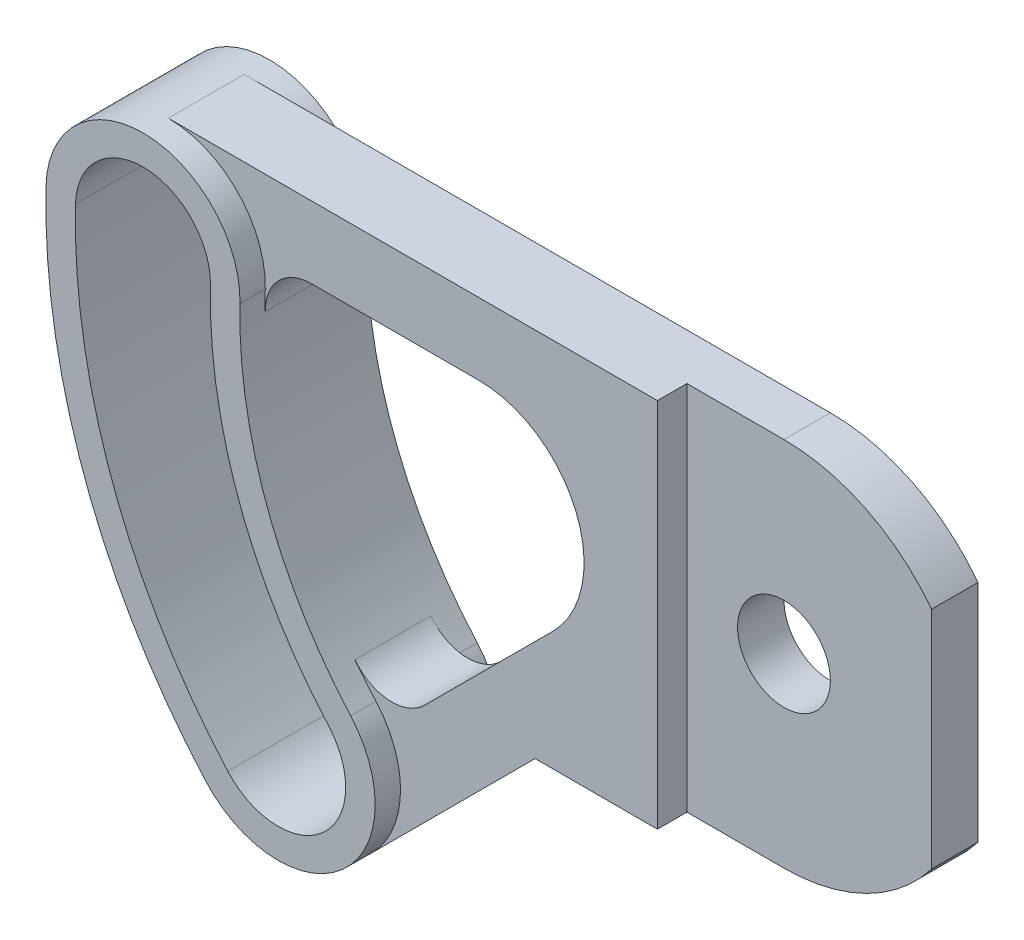
ISO-10303-21;
HEADER;
FILE_DESCRIPTION(('STEP AP214'),'2;1');
FILE_NAME('part.step','',(''),(''),'','','');
FILE_SCHEMA(('AUTOMOTIVE_DESIGN { 1 0 10303 214 1 1 1 1 }'));
ENDSEC;
DATA;
#1=APPLICATION_CONTEXT('core data for automotive mechanical design processes');
#2=APPLICATION_PROTOCOL_DEFINITION('international standard','automotive_design',2000,#1);
#3=PRODUCT_CONTEXT('',#1,'mechanical');
#4=PRODUCT('Part','Part','',(#3));
#5=PRODUCT_RELATED_PRODUCT_CATEGORY('part','',(#4));
#6=PRODUCT_DEFINITION_FORMATION('','',#4);
#7=PRODUCT_DEFINITION_CONTEXT('part definition',#1,'design');
#8=PRODUCT_DEFINITION('design','',#6,#7);
#9=PRODUCT_DEFINITION_SHAPE('','',#8);
#10=(LENGTH_UNIT() NAMED_UNIT(*) SI_UNIT(.MILLI.,.METRE.));
#11=(NAMED_UNIT(*) PLANE_ANGLE_UNIT() SI_UNIT($,.RADIAN.));
#12=(NAMED_UNIT(*) SI_UNIT($,.STERADIAN.) SOLID_ANGLE_UNIT());
#13=UNCERTAINTY_MEASURE_WITH_UNIT(LENGTH_MEASURE(1.E-05),#10,'distance_accuracy_value','');
#14=(GEOMETRIC_REPRESENTATION_CONTEXT(3) GLOBAL_UNCERTAINTY_ASSIGNED_CONTEXT((#13)) GLOBAL_UNIT_ASSIGNED_CONTEXT((#10,
#11,#12)) REPRESENTATION_CONTEXT('',''));
#15=CARTESIAN_POINT('',(0.,0.,0.));
#16=DIRECTION('',(0.,0.,1.));
#17=DIRECTION('',(1.,0.,0.));
#18=AXIS2_PLACEMENT_3D('',#15,#16,#17);
#19=CARTESIAN_POINT('',(-12.,18.,15.));
#20=DIRECTION('',(0.,0.,-1.));
#21=DIRECTION('',(-1.,0.,0.));
#22=AXIS2_PLACEMENT_3D('',#19,#20,#21);
#23=CYLINDRICAL_SURFACE('',#22,150.);
#24=CARTESIAN_POINT('',(-12.,18.,-15.));
#25=DIRECTION('',(0.,0.,1.));
#26=DIRECTION('',(1.,0.,0.));
#27=AXIS2_PLACEMENT_3D('',#24,#25,#26);
#28=CIRCLE('',#27,150.);
#29=CARTESIAN_POINT('',(-161.958144076572,21.5433070866141,-15.));
#30=VERTEX_POINT('',#29);
#31=CARTESIAN_POINT('',(-124.100356479706,-81.6669959270509,-15.));
#32=VERTEX_POINT('',#31);
#33=EDGE_CURVE('E384',#30,#32,#28,.T.);
#34=ORIENTED_EDGE('',*,*,#33,.T.);
#35=DIRECTION('',(0.,0.,-1.));
#36=VECTOR('',#35,1.);
#37=CARTESIAN_POINT('',(-124.100356479706,-81.6669959270509,15.));
#38=LINE('',#37,#36);
#39=CARTESIAN_POINT('',(-124.100356479706,-81.6669959270509,15.));
#40=VERTEX_POINT('',#39);
#41=EDGE_CURVE('E11',#40,#32,#38,.T.);
#42=ORIENTED_EDGE('',*,*,#41,.F.);
#43=CARTESIAN_POINT('',(-12.,18.,15.));
#44=DIRECTION('',(0.,0.,1.));
#45=DIRECTION('',(1.,0.,0.));
#46=AXIS2_PLACEMENT_3D('',#43,#44,#45);
#47=CIRCLE('',#46,150.);
#48=CARTESIAN_POINT('',(-161.958144076572,21.5433070866141,15.));
#49=VERTEX_POINT('',#48);
#50=EDGE_CURVE('E361',#49,#40,#47,.T.);
#51=ORIENTED_EDGE('',*,*,#50,.F.);
#52=DIRECTION('',(0.,0.,-1.));
#53=VECTOR('',#52,1.);
#54=CARTESIAN_POINT('',(-161.958144076572,21.5433070866141,15.));
#55=LINE('',#54,#53);
#56=EDGE_CURVE('E391',#49,#30,#55,.T.);
#57=ORIENTED_EDGE('',*,*,#56,.T.);
#58=EDGE_LOOP('',(#34,#42,#51,#57));
#59=FACE_BOUND('',#58,.T.);
#60=ADVANCED_FACE('F41',(#59),#23,.T.);
#61=CARTESIAN_POINT('',(-106.911635152818,-66.3847232182364,15.));
#62=DIRECTION('',(0.,0.,-1.));
#63=DIRECTION('',(-1.,0.,0.));
#64=AXIS2_PLACEMENT_3D('',#61,#62,#63);
#65=CYLINDRICAL_SURFACE('',#64,23.);
#66=DIRECTION('',(0.,0.,-1.));
#67=VECTOR('',#66,1.);
#68=CARTESIAN_POINT('',(-90.6481791855276,-82.6481791855272,9.));
#69=LINE('',#68,#67);
#70=CARTESIAN_POINT('',(-90.6481791855276,-82.6481791855272,9.));
#71=VERTEX_POINT('',#70);
#72=CARTESIAN_POINT('',(-90.6481791855276,-82.6481791855272,-9.));
#73=VERTEX_POINT('',#72);
#74=EDGE_CURVE('E343',#71,#73,#69,.T.);
#75=ORIENTED_EDGE('',*,*,#74,.F.);
#76=CARTESIAN_POINT('',(-106.911635152818,-66.3847232182364,9.));
#77=DIRECTION('',(0.,0.,1.));
#78=DIRECTION('',(1.,0.,0.));
#79=AXIS2_PLACEMENT_3D('',#76,#77,#78);
#80=CIRCLE('',#79,23.);
#81=CARTESIAN_POINT('',(-89.7229138259297,-51.1024505094219,9.));
#82=VERTEX_POINT('',#81);
#83=EDGE_CURVE('E272',#71,#82,#80,.T.);
#84=ORIENTED_EDGE('',*,*,#83,.T.);
#85=DIRECTION('',(0.,0.,-1.));
#86=VECTOR('',#85,1.);
#87=CARTESIAN_POINT('',(-89.7229138259297,-51.1024505094219,15.));
#88=LINE('',#87,#86);
#89=CARTESIAN_POINT('',(-89.7229138259297,-51.1024505094219,15.));
#90=VERTEX_POINT('',#89);
#91=EDGE_CURVE('E49',#90,#82,#88,.T.);
#92=ORIENTED_EDGE('',*,*,#91,.F.);
#93=CARTESIAN_POINT('',(-106.911635152818,-66.3847232182364,15.));
#94=DIRECTION('',(0.,0.,1.));
#95=DIRECTION('',(1.,0.,0.));
#96=AXIS2_PLACEMENT_3D('',#93,#94,#95);
#97=CIRCLE('',#96,23.);
#98=EDGE_CURVE('E368',#40,#90,#97,.T.);
#99=ORIENTED_EDGE('',*,*,#98,.F.);
#100=ORIENTED_EDGE('',*,*,#41,.T.);
#101=CARTESIAN_POINT('',(-106.911635152818,-66.3847232182364,-15.));
#102=DIRECTION('',(0.,0.,1.));
#103=DIRECTION('',(1.,0.,0.));
#104=AXIS2_PLACEMENT_3D('',#101,#102,#103);
#105=CIRCLE('',#104,23.);
#106=CARTESIAN_POINT('',(-89.7229138259297,-51.1024505094219,-15.));
#107=VERTEX_POINT('',#106);
#108=EDGE_CURVE('E389',#32,#107,#105,.T.);
#109=ORIENTED_EDGE('',*,*,#108,.T.);
#110=CARTESIAN_POINT('',(-89.7229138259297,-51.1024505094219,-9.));
#111=VERTEX_POINT('',#110);
#112=EDGE_CURVE('E405',#111,#107,#88,.T.);
#113=ORIENTED_EDGE('',*,*,#112,.F.);
#114=CARTESIAN_POINT('',(-106.911635152818,-66.3847232182364,-9.));
#115=DIRECTION('',(0.,0.,1.));
#116=DIRECTION('',(1.,0.,0.));
#117=AXIS2_PLACEMENT_3D('',#114,#115,#116);
#118=CIRCLE('',#117,23.);
#119=EDGE_CURVE('E310',#73,#111,#118,.T.);
#120=ORIENTED_EDGE('',*,*,#119,.F.);
#121=EDGE_LOOP('',(#75,#84,#92,#99,#100,#109,#113,#120));
#122=FACE_BOUND('',#121,.T.);
#123=ADVANCED_FACE('F436',(#122),#65,.T.);
#124=CARTESIAN_POINT('',(-12.,18.,15.));
#125=DIRECTION('',(0.,0.,-1.));
#126=DIRECTION('',(-1.,0.,0.));
#127=AXIS2_PLACEMENT_3D('',#124,#125,#126);
#128=CYLINDRICAL_SURFACE('',#127,104.);
#129=CARTESIAN_POINT('',(-12.,18.,9.));
#130=DIRECTION('',(0.,0.,1.));
#131=DIRECTION('',(1.,0.,0.));
#132=AXIS2_PLACEMENT_3D('',#129,#130,#131);
#133=CIRCLE('',#132,104.);
#134=CARTESIAN_POINT('',(-115.97097989309,20.4566929133858,9.));
#135=VERTEX_POINT('',#134);
#136=CARTESIAN_POINT('',(-115.975948195793,15.763440860215,9.));
#137=VERTEX_POINT('',#136);
#138=EDGE_CURVE('E273',#135,#137,#133,.T.);
#139=ORIENTED_EDGE('',*,*,#138,.F.);
#140=DIRECTION('',(0.,0.,-1.));
#141=VECTOR('',#140,1.);
#142=CARTESIAN_POINT('',(-115.97097989309,20.4566929133858,15.));
#143=LINE('',#142,#141);
#144=CARTESIAN_POINT('',(-115.97097989309,20.4566929133858,15.));
#145=VERTEX_POINT('',#144);
#146=EDGE_CURVE('E400',#145,#135,#143,.T.);
#147=ORIENTED_EDGE('',*,*,#146,.F.);
#148=CARTESIAN_POINT('',(-12.,18.,15.));
#149=DIRECTION('',(0.,0.,1.));
#150=DIRECTION('',(1.,0.,0.));
#151=AXIS2_PLACEMENT_3D('',#148,#149,#150);
#152=CIRCLE('',#151,104.);
#153=EDGE_CURVE('E366',#145,#90,#152,.T.);
#154=ORIENTED_EDGE('',*,*,#153,.T.);
#155=ORIENTED_EDGE('',*,*,#91,.T.);
#156=CARTESIAN_POINT('',(-94.7175715607182,-45.0381103388852,9.));
#157=VERTEX_POINT('',#156);
#158=EDGE_CURVE('E271',#157,#82,#133,.T.);
#159=ORIENTED_EDGE('',*,*,#158,.F.);
#160=DIRECTION('',(0.,0.,-1.));
#161=VECTOR('',#160,1.);
#162=CARTESIAN_POINT('',(-94.7175715607182,-45.0381103388852,9.));
#163=LINE('',#162,#161);
#164=CARTESIAN_POINT('',(-94.7175715607182,-45.0381103388852,-9.));
#165=VERTEX_POINT('',#164);
#166=EDGE_CURVE('E342',#157,#165,#163,.T.);
#167=ORIENTED_EDGE('',*,*,#166,.T.);
#168=CARTESIAN_POINT('',(-12.,18.,-9.));
#169=DIRECTION('',(0.,0.,1.));
#170=DIRECTION('',(1.,0.,0.));
#171=AXIS2_PLACEMENT_3D('',#168,#169,#170);
#172=CIRCLE('',#171,104.);
#173=EDGE_CURVE('E308',#165,#111,#172,.T.);
#174=ORIENTED_EDGE('',*,*,#173,.T.);
#175=ORIENTED_EDGE('',*,*,#112,.T.);
#176=CARTESIAN_POINT('',(-12.,18.,-15.));
#177=DIRECTION('',(0.,0.,1.));
#178=DIRECTION('',(1.,0.,0.));
#179=AXIS2_PLACEMENT_3D('',#176,#177,#178);
#180=CIRCLE('',#179,104.);
#181=CARTESIAN_POINT('',(-115.97097989309,20.4566929133858,-15.));
#182=VERTEX_POINT('',#181);
#183=EDGE_CURVE('E393',#182,#107,#180,.T.);
#184=ORIENTED_EDGE('',*,*,#183,.F.);
#185=CARTESIAN_POINT('',(-115.97097989309,20.4566929133858,-9.));
#186=VERTEX_POINT('',#185);
#187=EDGE_CURVE('E397',#186,#182,#143,.T.);
#188=ORIENTED_EDGE('',*,*,#187,.F.);
#189=CARTESIAN_POINT('',(-115.975948195793,15.763440860215,-9.));
#190=VERTEX_POINT('',#189);
#191=EDGE_CURVE('E309',#186,#190,#172,.T.);
#192=ORIENTED_EDGE('',*,*,#191,.T.);
#193=DIRECTION('',(0.,0.,-1.));
#194=VECTOR('',#193,1.);
#195=CARTESIAN_POINT('',(-115.975948195793,15.763440860215,9.));
#196=LINE('',#195,#194);
#197=EDGE_CURVE('E68',#137,#190,#196,.T.);
#198=ORIENTED_EDGE('',*,*,#197,.F.);
#199=EDGE_LOOP('',(#139,#147,#154,#155,#159,#167,#174,#175,#184,#188,#192,#198));
#200=FACE_BOUND('',#199,.T.);
#201=ADVANCED_FACE('F444',(#200),#128,.F.);
#202=CARTESIAN_POINT('',(-138.964561984831,20.9999999999999,15.));
#203=DIRECTION('',(0.,0.,-1.));
#204=DIRECTION('',(-1.,0.,0.));
#205=AXIS2_PLACEMENT_3D('',#202,#203,#204);
#206=CYLINDRICAL_SURFACE('',#205,16.);
#207=CARTESIAN_POINT('',(-138.964561984831,20.9999999999999,-15.));
#208=DIRECTION('',(0.,0.,1.));
#209=DIRECTION('',(1.,0.,0.));
#210=AXIS2_PLACEMENT_3D('',#207,#208,#209);
#211=CIRCLE('',#210,16.);
#212=CARTESIAN_POINT('',(-122.969026616663,20.6220472440944,-15.));
#213=VERTEX_POINT('',#212);
#214=CARTESIAN_POINT('',(-154.960097352999,21.3779527559055,-15.));
#215=VERTEX_POINT('',#214);
#216=EDGE_CURVE('E348',#213,#215,#211,.T.);
#217=ORIENTED_EDGE('',*,*,#216,.F.);
#218=DIRECTION('',(0.,0.,-1.));
#219=VECTOR('',#218,1.);
#220=CARTESIAN_POINT('',(-122.969026616663,20.6220472440944,15.));
#221=LINE('',#220,#219);
#222=CARTESIAN_POINT('',(-122.969026616663,20.6220472440944,15.));
#223=VERTEX_POINT('',#222);
#224=EDGE_CURVE('E44',#223,#213,#221,.T.);
#225=ORIENTED_EDGE('',*,*,#224,.F.);
#226=CARTESIAN_POINT('',(-138.964561984831,20.9999999999999,15.));
#227=DIRECTION('',(0.,0.,1.));
#228=DIRECTION('',(1.,0.,0.));
#229=AXIS2_PLACEMENT_3D('',#226,#227,#228);
#230=CIRCLE('',#229,16.);
#231=CARTESIAN_POINT('',(-154.960097352999,21.3779527559055,15.));
#232=VERTEX_POINT('',#231);
#233=EDGE_CURVE('E353',#223,#232,#230,.T.);
#234=ORIENTED_EDGE('',*,*,#233,.T.);
#235=DIRECTION('',(0.,0.,-1.));
#236=VECTOR('',#235,1.);
#237=CARTESIAN_POINT('',(-154.960097352999,21.3779527559055,15.));
#238=LINE('',#237,#236);
#239=EDGE_CURVE('E373',#232,#215,#238,.T.);
#240=ORIENTED_EDGE('',*,*,#239,.T.);
#241=EDGE_LOOP('',(#217,#225,#234,#240));
#242=FACE_BOUND('',#241,.T.);
#243=ADVANCED_FACE('F43',(#242),#206,.F.);
#244=CARTESIAN_POINT('',(-12.,18.,15.));
#245=DIRECTION('',(0.,0.,-1.));
#246=DIRECTION('',(-1.,0.,0.));
#247=AXIS2_PLACEMENT_3D('',#244,#245,#246);
#248=CYLINDRICAL_SURFACE('',#247,111.);
#249=CARTESIAN_POINT('',(-12.,18.,-15.));
#250=DIRECTION('',(0.,0.,1.));
#251=DIRECTION('',(1.,0.,0.));
#252=AXIS2_PLACEMENT_3D('',#249,#250,#251);
#253=CIRCLE('',#252,111.);
#254=CARTESIAN_POINT('',(-94.9542637949828,-55.7535769860178,-15.));
#255=VERTEX_POINT('',#254);
#256=EDGE_CURVE('E376',#213,#255,#253,.T.);
#257=ORIENTED_EDGE('',*,*,#256,.T.);
#258=DIRECTION('',(0.,0.,-1.));
#259=VECTOR('',#258,1.);
#260=CARTESIAN_POINT('',(-94.9542637949828,-55.7535769860178,15.));
#261=LINE('',#260,#259);
#262=CARTESIAN_POINT('',(-94.9542637949828,-55.7535769860178,15.));
#263=VERTEX_POINT('',#262);
#264=EDGE_CURVE('E409',#263,#255,#261,.T.);
#265=ORIENTED_EDGE('',*,*,#264,.F.);
#266=CARTESIAN_POINT('',(-12.,18.,15.));
#267=DIRECTION('',(0.,0.,1.));
#268=DIRECTION('',(1.,0.,0.));
#269=AXIS2_PLACEMENT_3D('',#266,#267,#268);
#270=CIRCLE('',#269,111.);
#271=EDGE_CURVE('E355',#223,#263,#270,.T.);
#272=ORIENTED_EDGE('',*,*,#271,.F.);
#273=ORIENTED_EDGE('',*,*,#224,.T.);
#274=EDGE_LOOP('',(#257,#265,#272,#273));
#275=FACE_BOUND('',#274,.T.);
#276=ADVANCED_FACE('F415',(#275),#248,.T.);
#277=CARTESIAN_POINT('',(-106.911635152818,-66.3847232182365,15.));
#278=DIRECTION('',(0.,0.,-1.));
#279=DIRECTION('',(-1.,0.,0.));
#280=AXIS2_PLACEMENT_3D('',#277,#278,#279);
#281=CYLINDRICAL_SURFACE('',#280,15.9999999999999);
#282=CARTESIAN_POINT('',(-106.911635152818,-66.3847232182365,-15.));
#283=DIRECTION('',(0.,0.,1.));
#284=DIRECTION('',(1.,0.,0.));
#285=AXIS2_PLACEMENT_3D('',#282,#283,#284);
#286=CIRCLE('',#285,15.9999999999999);
#287=CARTESIAN_POINT('',(-118.869006510653,-77.0158694504551,-15.));
#288=VERTEX_POINT('',#287);
#289=EDGE_CURVE('E377',#288,#255,#286,.T.);
#290=ORIENTED_EDGE('',*,*,#289,.F.);
#291=DIRECTION('',(0.,0.,-1.));
#292=VECTOR('',#291,1.);
#293=CARTESIAN_POINT('',(-118.869006510653,-77.0158694504551,15.));
#294=LINE('',#293,#292);
#295=CARTESIAN_POINT('',(-118.869006510653,-77.0158694504551,15.));
#296=VERTEX_POINT('',#295);
#297=EDGE_CURVE('E408',#296,#288,#294,.T.);
#298=ORIENTED_EDGE('',*,*,#297,.F.);
#299=CARTESIAN_POINT('',(-106.911635152818,-66.3847232182365,15.));
#300=DIRECTION('',(0.,0.,1.));
#301=DIRECTION('',(1.,0.,0.));
#302=AXIS2_PLACEMENT_3D('',#299,#300,#301);
#303=CIRCLE('',#302,15.9999999999999);
#304=EDGE_CURVE('E359',#296,#263,#303,.T.);
#305=ORIENTED_EDGE('',*,*,#304,.T.);
#306=ORIENTED_EDGE('',*,*,#264,.T.);
#307=EDGE_LOOP('',(#290,#298,#305,#306));
#308=FACE_BOUND('',#307,.T.);
#309=ADVANCED_FACE('F426',(#308),#281,.F.);
#310=CARTESIAN_POINT('',(-12.,18.,15.));
#311=DIRECTION('',(0.,0.,-1.));
#312=DIRECTION('',(-1.,0.,0.));
#313=AXIS2_PLACEMENT_3D('',#310,#311,#312);
#314=CYLINDRICAL_SURFACE('',#313,143.);
#315=CARTESIAN_POINT('',(-12.,18.,-15.));
#316=DIRECTION('',(0.,0.,1.));
#317=DIRECTION('',(1.,0.,0.));
#318=AXIS2_PLACEMENT_3D('',#315,#316,#317);
#319=CIRCLE('',#318,143.);
#320=EDGE_CURVE('E385',#215,#288,#319,.T.);
#321=ORIENTED_EDGE('',*,*,#320,.F.);
#322=ORIENTED_EDGE('',*,*,#239,.F.);
#323=CARTESIAN_POINT('',(-12.,18.,15.));
#324=DIRECTION('',(0.,0.,1.));
#325=DIRECTION('',(1.,0.,0.));
#326=AXIS2_PLACEMENT_3D('',#323,#324,#325);
#327=CIRCLE('',#326,143.);
#328=EDGE_CURVE('E356',#232,#296,#327,.T.);
#329=ORIENTED_EDGE('',*,*,#328,.T.);
#330=ORIENTED_EDGE('',*,*,#297,.T.);
#331=EDGE_LOOP('',(#321,#322,#329,#330));
#332=FACE_BOUND('',#331,.T.);
#333=ADVANCED_FACE('F424',(#332),#314,.F.);
#334=CARTESIAN_POINT('',(-138.964561984831,20.9999999999999,15.));
#335=DIRECTION('',(0.,0.,-1.));
#336=DIRECTION('',(-1.,0.,0.));
#337=AXIS2_PLACEMENT_3D('',#334,#335,#336);
#338=CYLINDRICAL_SURFACE('',#337,23.);
#339=ORIENTED_EDGE('',*,*,#146,.T.);
#340=CARTESIAN_POINT('',(-138.964561984831,20.9999999999999,9.));
#341=DIRECTION('',(0.,0.,1.));
#342=DIRECTION('',(1.,0.,0.));
#343=AXIS2_PLACEMENT_3D('',#340,#341,#342);
#344=CIRCLE('',#343,23.);
#345=CARTESIAN_POINT('',(-138.964561984831,44.,9.));
#346=VERTEX_POINT('',#345);
#347=EDGE_CURVE('E290',#135,#346,#344,.T.);
#348=ORIENTED_EDGE('',*,*,#347,.T.);
#349=DIRECTION('',(0.,0.,-1.));
#350=VECTOR('',#349,1.);
#351=CARTESIAN_POINT('',(-138.964561984831,44.,9.));
#352=LINE('',#351,#350);
#353=CARTESIAN_POINT('',(-138.964561984831,44.,-9.));
#354=VERTEX_POINT('',#353);
#355=EDGE_CURVE('E334',#346,#354,#352,.T.);
#356=ORIENTED_EDGE('',*,*,#355,.T.);
#357=CARTESIAN_POINT('',(-138.964561984831,20.9999999999999,-9.));
#358=DIRECTION('',(0.,0.,1.));
#359=DIRECTION('',(1.,0.,0.));
#360=AXIS2_PLACEMENT_3D('',#357,#358,#359);
#361=CIRCLE('',#360,23.);
#362=EDGE_CURVE('E321',#186,#354,#361,.T.);
#363=ORIENTED_EDGE('',*,*,#362,.F.);
#364=ORIENTED_EDGE('',*,*,#187,.T.);
#365=CARTESIAN_POINT('',(-138.964561984831,20.9999999999999,-15.));
#366=DIRECTION('',(0.,0.,1.));
#367=DIRECTION('',(1.,0.,0.));
#368=AXIS2_PLACEMENT_3D('',#365,#366,#367);
#369=CIRCLE('',#368,23.);
#370=EDGE_CURVE('E351',#182,#30,#369,.T.);
#371=ORIENTED_EDGE('',*,*,#370,.T.);
#372=ORIENTED_EDGE('',*,*,#56,.F.);
#373=CARTESIAN_POINT('',(-138.964561984831,20.9999999999999,15.));
#374=DIRECTION('',(0.,0.,1.));
#375=DIRECTION('',(1.,0.,0.));
#376=AXIS2_PLACEMENT_3D('',#373,#374,#375);
#377=CIRCLE('',#376,23.);
#378=EDGE_CURVE('E371',#145,#49,#377,.T.);
#379=ORIENTED_EDGE('',*,*,#378,.F.);
#380=EDGE_LOOP('',(#339,#348,#356,#363,#364,#371,#372,#379));
#381=FACE_BOUND('',#380,.T.);
#382=ADVANCED_FACE('F433',(#381),#338,.T.);
#383=CARTESIAN_POINT('',(0.,0.,15.));
#384=DIRECTION('',(0.,0.,1.));
#385=DIRECTION('',(1.,0.,0.));
#386=AXIS2_PLACEMENT_3D('',#383,#384,#385);
#387=PLANE('',#386);
#388=ORIENTED_EDGE('',*,*,#233,.F.);
#389=ORIENTED_EDGE('',*,*,#271,.T.);
#390=ORIENTED_EDGE('',*,*,#304,.F.);
#391=ORIENTED_EDGE('',*,*,#328,.F.);
#392=EDGE_LOOP('',(#388,#389,#390,#391));
#393=FACE_BOUND('',#392,.T.);
#394=ORIENTED_EDGE('',*,*,#50,.T.);
#395=ORIENTED_EDGE('',*,*,#98,.T.);
#396=ORIENTED_EDGE('',*,*,#153,.F.);
#397=ORIENTED_EDGE('',*,*,#378,.T.);
#398=EDGE_LOOP('',(#394,#395,#396,#397));
#399=FACE_BOUND('',#398,.T.);
#400=ADVANCED_FACE('F453',(#393,#399),#387,.T.);
#401=CARTESIAN_POINT('',(0.,0.,-15.));
#402=DIRECTION('',(0.,0.,1.));
#403=DIRECTION('',(1.,0.,0.));
#404=AXIS2_PLACEMENT_3D('',#401,#402,#403);
#405=PLANE('',#404);
#406=ORIENTED_EDGE('',*,*,#216,.T.);
#407=ORIENTED_EDGE('',*,*,#320,.T.);
#408=ORIENTED_EDGE('',*,*,#289,.T.);
#409=ORIENTED_EDGE('',*,*,#256,.F.);
#410=EDGE_LOOP('',(#406,#407,#408,#409));
#411=FACE_BOUND('',#410,.T.);
#412=ORIENTED_EDGE('',*,*,#33,.F.);
#413=ORIENTED_EDGE('',*,*,#370,.F.);
#414=ORIENTED_EDGE('',*,*,#183,.T.);
#415=ORIENTED_EDGE('',*,*,#108,.F.);
#416=EDGE_LOOP('',(#412,#413,#414,#415));
#417=FACE_BOUND('',#416,.T.);
#418=ADVANCED_FACE('F420',(#411,#417),#405,.F.);
#419=CARTESIAN_POINT('',(-65.3969696196698,1.99999999999999,9.));
#420=DIRECTION('',(0.,0.,-1.));
#421=DIRECTION('',(-1.,0.,0.));
#422=AXIS2_PLACEMENT_3D('',#419,#420,#421);
#423=CYLINDRICAL_SURFACE('',#422,25.);
#424=CARTESIAN_POINT('',(-65.3969696196698,1.99999999999999,-9.));
#425=DIRECTION('',(0.,0.,1.));
#426=DIRECTION('',(1.,0.,0.));
#427=AXIS2_PLACEMENT_3D('',#424,#425,#426);
#428=CIRCLE('',#427,25.);
#429=CARTESIAN_POINT('',(-47.7193000900062,-15.6776695296637,-9.));
#430=VERTEX_POINT('',#429);
#431=CARTESIAN_POINT('',(-65.3969696196698,27.,-9.));
#432=VERTEX_POINT('',#431);
#433=EDGE_CURVE('E256',#430,#432,#428,.T.);
#434=ORIENTED_EDGE('',*,*,#433,.F.);
#435=DIRECTION('',(0.,0.,-1.));
#436=VECTOR('',#435,1.);
#437=CARTESIAN_POINT('',(-47.7193000900062,-15.6776695296637,9.));
#438=LINE('',#437,#436);
#439=CARTESIAN_POINT('',(-47.7193000900062,-15.6776695296637,9.));
#440=VERTEX_POINT('',#439);
#441=EDGE_CURVE('E346',#440,#430,#438,.T.);
#442=ORIENTED_EDGE('',*,*,#441,.F.);
#443=CARTESIAN_POINT('',(-65.3969696196698,1.99999999999999,9.));
#444=DIRECTION('',(0.,0.,1.));
#445=DIRECTION('',(1.,0.,0.));
#446=AXIS2_PLACEMENT_3D('',#443,#444,#445);
#447=CIRCLE('',#446,25.);
#448=CARTESIAN_POINT('',(-65.3969696196698,27.,9.));
#449=VERTEX_POINT('',#448);
#450=EDGE_CURVE('E265',#440,#449,#447,.T.);
#451=ORIENTED_EDGE('',*,*,#450,.T.);
#452=DIRECTION('',(0.,0.,-1.));
#453=VECTOR('',#452,1.);
#454=CARTESIAN_POINT('',(-65.3969696196698,27.,9.));
#455=LINE('',#454,#453);
#456=EDGE_CURVE('E299',#449,#432,#455,.T.);
#457=ORIENTED_EDGE('',*,*,#456,.T.);
#458=EDGE_LOOP('',(#434,#442,#451,#457));
#459=FACE_BOUND('',#458,.T.);
#460=ADVANCED_FACE('F451',(#459),#423,.F.);
#461=CARTESIAN_POINT('',(-16.020815280171,16.0208152801712,9.));
#462=DIRECTION('',(0.707106781186544,-0.707106781186551,0.));
#463=DIRECTION('',(0.707106781186551,0.707106781186544,0.));
#464=AXIS2_PLACEMENT_3D('',#461,#462,#463);
#465=PLANE('',#464);
#466=DIRECTION('',(-0.707106781186551,-0.707106781186544,0.));
#467=VECTOR('',#466,1.);
#468=CARTESIAN_POINT('',(-16.020815280171,16.0208152801712,-9.));
#469=LINE('',#468,#467);
#470=CARTESIAN_POINT('',(-78.1904230525903,-46.1487924922475,-9.));
#471=VERTEX_POINT('',#470);
#472=EDGE_CURVE('E296',#430,#471,#469,.T.);
#473=ORIENTED_EDGE('',*,*,#472,.T.);
#474=DIRECTION('',(0.,0.,-1.));
#475=VECTOR('',#474,1.);
#476=CARTESIAN_POINT('',(-78.1904230525903,-46.1487924922475,9.));
#477=LINE('',#476,#475);
#478=CARTESIAN_POINT('',(-78.1904230525903,-46.1487924922475,9.));
#479=VERTEX_POINT('',#478);
#480=EDGE_CURVE('E347',#479,#471,#477,.T.);
#481=ORIENTED_EDGE('',*,*,#480,.F.);
#482=DIRECTION('',(-0.707106781186551,-0.707106781186544,0.));
#483=VECTOR('',#482,1.);
#484=CARTESIAN_POINT('',(-16.020815280171,16.0208152801712,9.));
#485=LINE('',#484,#483);
#486=EDGE_CURVE('E264',#440,#479,#485,.T.);
#487=ORIENTED_EDGE('',*,*,#486,.F.);
#488=ORIENTED_EDGE('',*,*,#441,.T.);
#489=EDGE_LOOP('',(#473,#481,#487,#488));
#490=FACE_BOUND('',#489,.T.);
#491=ADVANCED_FACE('F463',(#490),#465,.F.);
#492=CARTESIAN_POINT('',(-85.9685976456422,-38.3706178991954,9.));
#493=DIRECTION('',(0.,0.,-1.));
#494=DIRECTION('',(-1.,0.,0.));
#495=AXIS2_PLACEMENT_3D('',#492,#493,#494);
#496=CYLINDRICAL_SURFACE('',#495,11.);
#497=CARTESIAN_POINT('',(-85.9685976456422,-38.3706178991954,-9.));
#498=DIRECTION('',(0.,0.,1.));
#499=DIRECTION('',(1.,0.,0.));
#500=AXIS2_PLACEMENT_3D('',#497,#498,#499);
#501=CIRCLE('',#500,11.);
#502=EDGE_CURVE('E302',#165,#471,#501,.T.);
#503=ORIENTED_EDGE('',*,*,#502,.F.);
#504=ORIENTED_EDGE('',*,*,#166,.F.);
#505=CARTESIAN_POINT('',(-85.9685976456422,-38.3706178991954,9.));
#506=DIRECTION('',(0.,0.,1.));
#507=DIRECTION('',(1.,0.,0.));
#508=AXIS2_PLACEMENT_3D('',#505,#506,#507);
#509=CIRCLE('',#508,11.);
#510=EDGE_CURVE('E268',#157,#479,#509,.T.);
#511=ORIENTED_EDGE('',*,*,#510,.T.);
#512=ORIENTED_EDGE('',*,*,#480,.T.);
#513=EDGE_LOOP('',(#503,#504,#511,#512));
#514=FACE_BOUND('',#513,.T.);
#515=ADVANCED_FACE('F461',(#514),#496,.F.);
#516=CARTESIAN_POINT('',(-3.99999999999973,3.99999999999977,9.));
#517=DIRECTION('',(0.707106781186544,-0.707106781186551,0.));
#518=DIRECTION('',(0.707106781186551,0.707106781186544,0.));
#519=AXIS2_PLACEMENT_3D('',#516,#517,#518);
#520=PLANE('',#519);
#521=DIRECTION('',(-0.707106781186551,-0.707106781186544,0.));
#522=VECTOR('',#521,1.);
#523=CARTESIAN_POINT('',(-3.99999999999973,3.99999999999977,-9.));
#524=LINE('',#523,#522);
#525=CARTESIAN_POINT('',(-52.,-44.,-9.));
#526=VERTEX_POINT('',#525);
#527=EDGE_CURVE('E315',#526,#73,#524,.T.);
#528=ORIENTED_EDGE('',*,*,#527,.F.);
#529=DIRECTION('',(0.,0.,-1.));
#530=VECTOR('',#529,1.);
#531=CARTESIAN_POINT('',(-52.,-44.,9.));
#532=LINE('',#531,#530);
#533=CARTESIAN_POINT('',(-52.,-44.,9.));
#534=VERTEX_POINT('',#533);
#535=EDGE_CURVE('E340',#534,#526,#532,.T.);
#536=ORIENTED_EDGE('',*,*,#535,.F.);
#537=DIRECTION('',(-0.707106781186551,-0.707106781186544,0.));
#538=VECTOR('',#537,1.);
#539=CARTESIAN_POINT('',(-3.99999999999973,3.99999999999977,9.));
#540=LINE('',#539,#538);
#541=EDGE_CURVE('E280',#534,#71,#540,.T.);
#542=ORIENTED_EDGE('',*,*,#541,.T.);
#543=ORIENTED_EDGE('',*,*,#74,.T.);
#544=EDGE_LOOP('',(#528,#536,#542,#543));
#545=FACE_BOUND('',#544,.T.);
#546=ADVANCED_FACE('F470',(#545),#520,.T.);
#547=CARTESIAN_POINT('',(0.,-44.,9.));
#548=DIRECTION('',(0.,-1.,0.));
#549=DIRECTION('',(0.,0.,-1.));
#550=AXIS2_PLACEMENT_3D('',#547,#548,#549);
#551=PLANE('',#550);
#552=DIRECTION('',(-1.,0.,0.));
#553=VECTOR('',#552,1.);
#554=CARTESIAN_POINT('',(0.,-44.,-9.));
#555=LINE('',#554,#553);
#556=CARTESIAN_POINT('',(0.,-44.,-9.));
#557=VERTEX_POINT('',#556);
#558=EDGE_CURVE('E312',#557,#526,#555,.T.);
#559=ORIENTED_EDGE('',*,*,#558,.F.);
#560=DIRECTION('',(0.,0.,1.));
#561=VECTOR('',#560,1.);
#562=CARTESIAN_POINT('',(0.,-44.,-9.));
#563=LINE('',#562,#561);
#564=CARTESIAN_POINT('',(0.,-44.,2.));
#565=VERTEX_POINT('',#564);
#566=EDGE_CURVE('E259',#557,#565,#563,.T.);
#567=ORIENTED_EDGE('',*,*,#566,.T.);
#568=DIRECTION('',(-1.,0.,0.));
#569=VECTOR('',#568,1.);
#570=CARTESIAN_POINT('',(0.,-44.,2.));
#571=LINE('',#570,#569);
#572=CARTESIAN_POINT('',(-23.,-44.,2.));
#573=VERTEX_POINT('',#572);
#574=EDGE_CURVE('E245',#565,#573,#571,.T.);
#575=ORIENTED_EDGE('',*,*,#574,.T.);
#576=DIRECTION('',(0.,0.,-1.));
#577=VECTOR('',#576,1.);
#578=CARTESIAN_POINT('',(-23.,-44.,9.));
#579=LINE('',#578,#577);
#580=CARTESIAN_POINT('',(-23.,-44.,9.));
#581=VERTEX_POINT('',#580);
#582=EDGE_CURVE('E339',#581,#573,#579,.T.);
#583=ORIENTED_EDGE('',*,*,#582,.F.);
#584=DIRECTION('',(-1.,0.,0.));
#585=VECTOR('',#584,1.);
#586=CARTESIAN_POINT('',(0.,-44.,9.));
#587=LINE('',#586,#585);
#588=EDGE_CURVE('E278',#581,#534,#587,.T.);
#589=ORIENTED_EDGE('',*,*,#588,.T.);
#590=ORIENTED_EDGE('',*,*,#535,.T.);
#591=EDGE_LOOP('',(#559,#567,#575,#583,#589,#590));
#592=FACE_BOUND('',#591,.T.);
#593=ADVANCED_FACE('F471',(#592),#551,.T.);
#594=CARTESIAN_POINT('',(-23.,0.,9.));
#595=DIRECTION('',(1.,0.,0.));
#596=DIRECTION('',(0.,1.,0.));
#597=AXIS2_PLACEMENT_3D('',#594,#595,#596);
#598=PLANE('',#597);
#599=DIRECTION('',(0.,-1.,0.));
#600=VECTOR('',#599,1.);
#601=CARTESIAN_POINT('',(-23.,0.,2.));
#602=LINE('',#601,#600);
#603=CARTESIAN_POINT('',(-23.,44.,2.));
#604=VERTEX_POINT('',#603);
#605=EDGE_CURVE('E59',#604,#573,#602,.T.);
#606=ORIENTED_EDGE('',*,*,#605,.F.);
#607=DIRECTION('',(0.,0.,-1.));
#608=VECTOR('',#607,1.);
#609=CARTESIAN_POINT('',(-23.,44.,9.));
#610=LINE('',#609,#608);
#611=CARTESIAN_POINT('',(-23.,44.,9.));
#612=VERTEX_POINT('',#611);
#613=EDGE_CURVE('E333',#612,#604,#610,.T.);
#614=ORIENTED_EDGE('',*,*,#613,.F.);
#615=DIRECTION('',(0.,-1.,0.));
#616=VECTOR('',#615,1.);
#617=CARTESIAN_POINT('',(-23.,0.,9.));
#618=LINE('',#617,#616);
#619=EDGE_CURVE('E282',#612,#581,#618,.T.);
#620=ORIENTED_EDGE('',*,*,#619,.T.);
#621=ORIENTED_EDGE('',*,*,#582,.T.);
#622=EDGE_LOOP('',(#606,#614,#620,#621));
#623=FACE_BOUND('',#622,.T.);
#624=ADVANCED_FACE('F480',(#623),#598,.T.);
#625=CARTESIAN_POINT('',(0.,44.,9.));
#626=DIRECTION('',(0.,-1.,0.));
#627=DIRECTION('',(0.,0.,-1.));
#628=AXIS2_PLACEMENT_3D('',#625,#626,#627);
#629=PLANE('',#628);
#630=DIRECTION('',(-1.,0.,0.));
#631=VECTOR('',#630,1.);
#632=CARTESIAN_POINT('',(0.,44.,-9.));
#633=LINE('',#632,#631);
#634=CARTESIAN_POINT('',(0.,44.,-9.));
#635=VERTEX_POINT('',#634);
#636=EDGE_CURVE('E318',#635,#354,#633,.T.);
#637=ORIENTED_EDGE('',*,*,#636,.T.);
#638=ORIENTED_EDGE('',*,*,#355,.F.);
#639=DIRECTION('',(-1.,0.,0.));
#640=VECTOR('',#639,1.);
#641=CARTESIAN_POINT('',(0.,44.,9.));
#642=LINE('',#641,#640);
#643=EDGE_CURVE('E288',#612,#346,#642,.T.);
#644=ORIENTED_EDGE('',*,*,#643,.F.);
#645=ORIENTED_EDGE('',*,*,#613,.T.);
#646=DIRECTION('',(-1.,0.,0.));
#647=VECTOR('',#646,1.);
#648=CARTESIAN_POINT('',(0.,44.,2.));
#649=LINE('',#648,#647);
#650=CARTESIAN_POINT('',(0.,44.,2.));
#651=VERTEX_POINT('',#650);
#652=EDGE_CURVE('E226',#651,#604,#649,.T.);
#653=ORIENTED_EDGE('',*,*,#652,.F.);
#654=DIRECTION('',(0.,0.,1.));
#655=VECTOR('',#654,1.);
#656=CARTESIAN_POINT('',(0.,44.,-9.));
#657=LINE('',#656,#655);
#658=EDGE_CURVE('E219',#635,#651,#657,.T.);
#659=ORIENTED_EDGE('',*,*,#658,.F.);
#660=EDGE_LOOP('',(#637,#638,#644,#645,#653,#659));
#661=FACE_BOUND('',#660,.T.);
#662=ADVANCED_FACE('F481',(#661),#629,.F.);
#663=CARTESIAN_POINT('',(-104.978492136623,16.,9.));
#664=DIRECTION('',(0.,0.,-1.));
#665=DIRECTION('',(-1.,0.,0.));
#666=AXIS2_PLACEMENT_3D('',#663,#664,#665);
#667=CYLINDRICAL_SURFACE('',#666,11.);
#668=CARTESIAN_POINT('',(-104.978492136623,16.,-9.));
#669=DIRECTION('',(0.,0.,1.));
#670=DIRECTION('',(1.,0.,0.));
#671=AXIS2_PLACEMENT_3D('',#668,#669,#670);
#672=CIRCLE('',#671,11.);
#673=CARTESIAN_POINT('',(-104.978492136623,27.,-9.));
#674=VERTEX_POINT('',#673);
#675=EDGE_CURVE('E322',#674,#190,#672,.T.);
#676=ORIENTED_EDGE('',*,*,#675,.F.);
#677=DIRECTION('',(0.,0.,-1.));
#678=VECTOR('',#677,1.);
#679=CARTESIAN_POINT('',(-104.978492136623,27.,9.));
#680=LINE('',#679,#678);
#681=CARTESIAN_POINT('',(-104.978492136623,27.,9.));
#682=VERTEX_POINT('',#681);
#683=EDGE_CURVE('E329',#682,#674,#680,.T.);
#684=ORIENTED_EDGE('',*,*,#683,.F.);
#685=CARTESIAN_POINT('',(-104.978492136623,16.,9.));
#686=DIRECTION('',(0.,0.,1.));
#687=DIRECTION('',(1.,0.,0.));
#688=AXIS2_PLACEMENT_3D('',#685,#686,#687);
#689=CIRCLE('',#688,11.);
#690=EDGE_CURVE('E292',#682,#137,#689,.T.);
#691=ORIENTED_EDGE('',*,*,#690,.T.);
#692=ORIENTED_EDGE('',*,*,#197,.T.);
#693=EDGE_LOOP('',(#676,#684,#691,#692));
#694=FACE_BOUND('',#693,.T.);
#695=ADVANCED_FACE('F482',(#694),#667,.F.);
#696=CARTESIAN_POINT('',(0.,27.,9.));
#697=DIRECTION('',(0.,-1.,0.));
#698=DIRECTION('',(1.,0.,0.));
#699=AXIS2_PLACEMENT_3D('',#696,#697,#698);
#700=PLANE('',#699);
#701=DIRECTION('',(-1.,0.,0.));
#702=VECTOR('',#701,1.);
#703=CARTESIAN_POINT('',(0.,27.,-9.));
#704=LINE('',#703,#702);
#705=EDGE_CURVE('E266',#432,#674,#704,.T.);
#706=ORIENTED_EDGE('',*,*,#705,.F.);
#707=ORIENTED_EDGE('',*,*,#456,.F.);
#708=DIRECTION('',(-1.,0.,0.));
#709=VECTOR('',#708,1.);
#710=CARTESIAN_POINT('',(0.,27.,9.));
#711=LINE('',#710,#709);
#712=EDGE_CURVE('E294',#449,#682,#711,.T.);
#713=ORIENTED_EDGE('',*,*,#712,.T.);
#714=ORIENTED_EDGE('',*,*,#683,.T.);
#715=EDGE_LOOP('',(#706,#707,#713,#714));
#716=FACE_BOUND('',#715,.T.);
#717=ADVANCED_FACE('F488',(#716),#700,.T.);
#718=CARTESIAN_POINT('',(0.,0.,9.));
#719=DIRECTION('',(0.,0.,1.));
#720=DIRECTION('',(1.,0.,0.));
#721=AXIS2_PLACEMENT_3D('',#718,#719,#720);
#722=PLANE('',#721);
#723=ORIENTED_EDGE('',*,*,#450,.F.);
#724=ORIENTED_EDGE('',*,*,#486,.T.);
#725=ORIENTED_EDGE('',*,*,#510,.F.);
#726=ORIENTED_EDGE('',*,*,#158,.T.);
#727=ORIENTED_EDGE('',*,*,#83,.F.);
#728=ORIENTED_EDGE('',*,*,#541,.F.);
#729=ORIENTED_EDGE('',*,*,#588,.F.);
#730=ORIENTED_EDGE('',*,*,#619,.F.);
#731=ORIENTED_EDGE('',*,*,#643,.T.);
#732=ORIENTED_EDGE('',*,*,#347,.F.);
#733=ORIENTED_EDGE('',*,*,#138,.T.);
#734=ORIENTED_EDGE('',*,*,#690,.F.);
#735=ORIENTED_EDGE('',*,*,#712,.F.);
#736=EDGE_LOOP('',(#723,#724,#725,#726,#727,#728,#729,#730,#731,#732,#733,#734,#735));
#737=FACE_BOUND('',#736,.T.);
#738=ADVANCED_FACE('F495',(#737),#722,.T.);
#739=CARTESIAN_POINT('',(0.,0.,-9.));
#740=DIRECTION('',(0.,0.,1.));
#741=DIRECTION('',(1.,0.,0.));
#742=AXIS2_PLACEMENT_3D('',#739,#740,#741);
#743=PLANE('',#742);
#744=ORIENTED_EDGE('',*,*,#433,.T.);
#745=ORIENTED_EDGE('',*,*,#705,.T.);
#746=ORIENTED_EDGE('',*,*,#675,.T.);
#747=ORIENTED_EDGE('',*,*,#191,.F.);
#748=ORIENTED_EDGE('',*,*,#362,.T.);
#749=ORIENTED_EDGE('',*,*,#636,.F.);
#750=CARTESIAN_POINT('',(0.,0.,-9.));
#751=DIRECTION('',(0.,0.,1.));
#752=DIRECTION('',(1.,0.,0.));
#753=AXIS2_PLACEMENT_3D('',#750,#751,#752);
#754=CIRCLE('',#753,44.);
#755=CARTESIAN_POINT('',(35.,26.6645832519468,-9.));
#756=VERTEX_POINT('',#755);
#757=EDGE_CURVE('E252',#756,#635,#754,.T.);
#758=ORIENTED_EDGE('',*,*,#757,.F.);
#759=DIRECTION('',(0.,-1.,0.));
#760=VECTOR('',#759,1.);
#761=CARTESIAN_POINT('',(35.,0.,-9.));
#762=LINE('',#761,#760);
#763=CARTESIAN_POINT('',(35.,-26.6645832519467,-9.));
#764=VERTEX_POINT('',#763);
#765=EDGE_CURVE('E216',#756,#764,#762,.T.);
#766=ORIENTED_EDGE('',*,*,#765,.T.);
#767=CARTESIAN_POINT('',(0.,0.,-9.));
#768=DIRECTION('',(0.,0.,1.));
#769=DIRECTION('',(1.,0.,0.));
#770=AXIS2_PLACEMENT_3D('',#767,#768,#769);
#771=CIRCLE('',#770,44.);
#772=EDGE_CURVE('E222',#557,#764,#771,.T.);
#773=ORIENTED_EDGE('',*,*,#772,.F.);
#774=ORIENTED_EDGE('',*,*,#558,.T.);
#775=ORIENTED_EDGE('',*,*,#527,.T.);
#776=ORIENTED_EDGE('',*,*,#119,.T.);
#777=ORIENTED_EDGE('',*,*,#173,.F.);
#778=ORIENTED_EDGE('',*,*,#502,.T.);
#779=ORIENTED_EDGE('',*,*,#472,.F.);
#780=EDGE_LOOP('',(#744,#745,#746,#747,#748,#749,#758,#766,#773,#774,#775,#776,#777,#778,#779));
#781=FACE_BOUND('',#780,.T.);
#782=CARTESIAN_POINT('',(0.,0.,-9.));
#783=DIRECTION('',(0.,0.,1.));
#784=DIRECTION('',(1.,0.,0.));
#785=AXIS2_PLACEMENT_3D('',#782,#783,#784);
#786=CIRCLE('',#785,11.);
#787=CARTESIAN_POINT('',(11.,0.,-9.));
#788=VERTEX_POINT('',#787);
#789=EDGE_CURVE('E247',#788,#788,#786,.T.);
#790=ORIENTED_EDGE('',*,*,#789,.T.);
#791=EDGE_LOOP('',(#790));
#792=FACE_BOUND('',#791,.T.);
#793=ADVANCED_FACE('F493',(#781,#792),#743,.F.);
#794=CARTESIAN_POINT('',(35.,0.,-9.));
#795=DIRECTION('',(-1.,0.,0.));
#796=DIRECTION('',(0.,0.,1.));
#797=AXIS2_PLACEMENT_3D('',#794,#795,#796);
#798=PLANE('',#797);
#799=DIRECTION('',(0.,0.,1.));
#800=VECTOR('',#799,1.);
#801=CARTESIAN_POINT('',(35.,26.6645832519468,-9.));
#802=LINE('',#801,#800);
#803=CARTESIAN_POINT('',(35.,26.6645832519468,2.));
#804=VERTEX_POINT('',#803);
#805=EDGE_CURVE('E209',#756,#804,#802,.T.);
#806=ORIENTED_EDGE('',*,*,#805,.T.);
#807=DIRECTION('',(0.,-1.,0.));
#808=VECTOR('',#807,1.);
#809=CARTESIAN_POINT('',(35.,0.,2.));
#810=LINE('',#809,#808);
#811=CARTESIAN_POINT('',(35.,-26.6645832519467,2.));
#812=VERTEX_POINT('',#811);
#813=EDGE_CURVE('E214',#804,#812,#810,.T.);
#814=ORIENTED_EDGE('',*,*,#813,.T.);
#815=DIRECTION('',(0.,0.,1.));
#816=VECTOR('',#815,1.);
#817=CARTESIAN_POINT('',(35.,-26.6645832519467,-9.));
#818=LINE('',#817,#816);
#819=EDGE_CURVE('E258',#764,#812,#818,.T.);
#820=ORIENTED_EDGE('',*,*,#819,.F.);
#821=ORIENTED_EDGE('',*,*,#765,.F.);
#822=EDGE_LOOP('',(#806,#814,#820,#821));
#823=FACE_BOUND('',#822,.T.);
#824=ADVANCED_FACE('F215',(#823),#798,.F.);
#825=CARTESIAN_POINT('',(0.,0.,-9.));
#826=DIRECTION('',(0.,0.,1.));
#827=DIRECTION('',(1.,0.,0.));
#828=AXIS2_PLACEMENT_3D('',#825,#826,#827);
#829=CYLINDRICAL_SURFACE('',#828,44.);
#830=ORIENTED_EDGE('',*,*,#819,.T.);
#831=CARTESIAN_POINT('',(0.,0.,2.));
#832=DIRECTION('',(0.,0.,1.));
#833=DIRECTION('',(1.,0.,0.));
#834=AXIS2_PLACEMENT_3D('',#831,#832,#833);
#835=CIRCLE('',#834,44.);
#836=EDGE_CURVE('E237',#565,#812,#835,.T.);
#837=ORIENTED_EDGE('',*,*,#836,.F.);
#838=ORIENTED_EDGE('',*,*,#566,.F.);
#839=ORIENTED_EDGE('',*,*,#772,.T.);
#840=EDGE_LOOP('',(#830,#837,#838,#839));
#841=FACE_BOUND('',#840,.T.);
#842=ADVANCED_FACE('F505',(#841),#829,.T.);
#843=CARTESIAN_POINT('',(0.,0.,-9.));
#844=DIRECTION('',(0.,0.,1.));
#845=DIRECTION('',(1.,0.,0.));
#846=AXIS2_PLACEMENT_3D('',#843,#844,#845);
#847=CYLINDRICAL_SURFACE('',#846,11.);
#848=ORIENTED_EDGE('',*,*,#789,.F.);
#849=EDGE_LOOP('',(#848));
#850=FACE_BOUND('',#849,.T.);
#851=CARTESIAN_POINT('',(0.,0.,2.));
#852=DIRECTION('',(0.,0.,1.));
#853=DIRECTION('',(1.,0.,0.));
#854=AXIS2_PLACEMENT_3D('',#851,#852,#853);
#855=CIRCLE('',#854,11.);
#856=CARTESIAN_POINT('',(11.,0.,2.));
#857=VERTEX_POINT('',#856);
#858=EDGE_CURVE('E240',#857,#857,#855,.T.);
#859=ORIENTED_EDGE('',*,*,#858,.T.);
#860=EDGE_LOOP('',(#859));
#861=FACE_BOUND('',#860,.T.);
#862=ADVANCED_FACE('F503',(#850,#861),#847,.F.);
#863=CARTESIAN_POINT('',(0.,0.,-9.));
#864=DIRECTION('',(0.,0.,1.));
#865=DIRECTION('',(1.,0.,0.));
#866=AXIS2_PLACEMENT_3D('',#863,#864,#865);
#867=CYLINDRICAL_SURFACE('',#866,44.);
#868=ORIENTED_EDGE('',*,*,#658,.T.);
#869=CARTESIAN_POINT('',(0.,0.,2.));
#870=DIRECTION('',(0.,0.,1.));
#871=DIRECTION('',(1.,0.,0.));
#872=AXIS2_PLACEMENT_3D('',#869,#870,#871);
#873=CIRCLE('',#872,44.);
#874=EDGE_CURVE('E221',#804,#651,#873,.T.);
#875=ORIENTED_EDGE('',*,*,#874,.F.);
#876=ORIENTED_EDGE('',*,*,#805,.F.);
#877=ORIENTED_EDGE('',*,*,#757,.T.);
#878=EDGE_LOOP('',(#868,#875,#876,#877));
#879=FACE_BOUND('',#878,.T.);
#880=ADVANCED_FACE('F223',(#879),#867,.T.);
#881=CARTESIAN_POINT('',(0.,0.,2.));
#882=DIRECTION('',(0.,0.,1.));
#883=DIRECTION('',(1.,0.,0.));
#884=AXIS2_PLACEMENT_3D('',#881,#882,#883);
#885=PLANE('',#884);
#886=ORIENTED_EDGE('',*,*,#858,.F.);
#887=EDGE_LOOP('',(#886));
#888=FACE_BOUND('',#887,.T.);
#889=ORIENTED_EDGE('',*,*,#813,.F.);
#890=ORIENTED_EDGE('',*,*,#874,.T.);
#891=ORIENTED_EDGE('',*,*,#652,.T.);
#892=ORIENTED_EDGE('',*,*,#605,.T.);
#893=ORIENTED_EDGE('',*,*,#574,.F.);
#894=ORIENTED_EDGE('',*,*,#836,.T.);
#895=EDGE_LOOP('',(#889,#890,#891,#892,#893,#894));
#896=FACE_BOUND('',#895,.T.);
#897=ADVANCED_FACE('F232',(#888,#896),#885,.T.);
#898=CLOSED_SHELL('',(#60,#123,#201,#243,#276,#309,#333,#382,#400,#418,#460,#491,#515,#546,#593,
#624,#662,#695,#717,#738,#793,#824,#842,#862,#880,#897));
#899=MANIFOLD_SOLID_BREP('B2',#898);
#900=ADVANCED_BREP_SHAPE_REPRESENTATION('',(#18,#899),#14);
#901=SHAPE_DEFINITION_REPRESENTATION(#9,#900);
ENDSEC;
END-ISO-10303-21;
